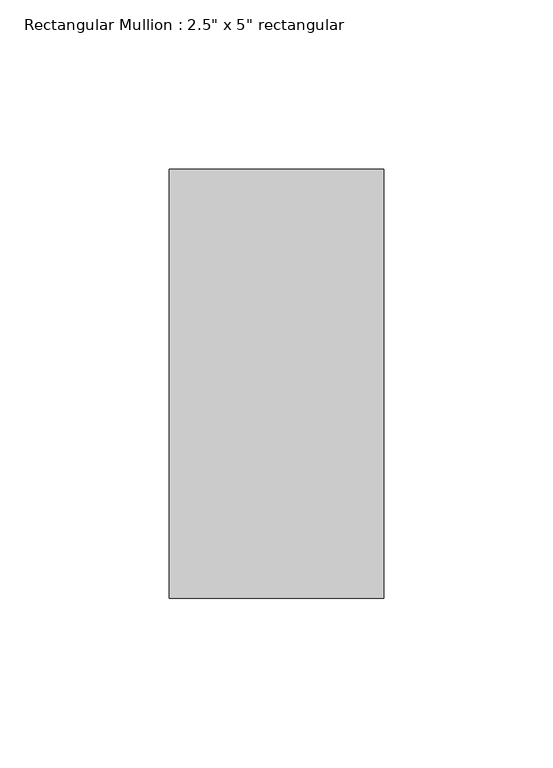
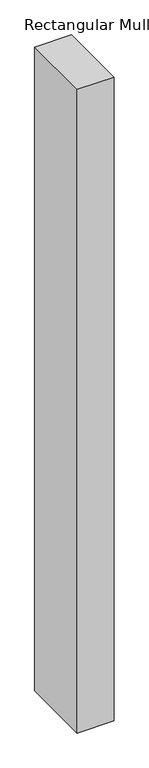
"""IFC4 building model written with IfcOpenShell, lengths in millimetres: member geometry."""

from ifc_helpers import new_model, si_unit, frame, origin, place, context, project, spatial, polyline, outline, extrude, source, transform, mapped, element, save


def member_7f2c8287(model_context):
    return source(origin(), model_context, "Body", "SweptSolid", [
        extrude(outline(polyline([(31.75, 63.5), (31.75, -63.5), (-31.75, -63.5), (-31.75, 63.5), (31.75, 63.5)])), frame((0.0, 0.0, -1174.7500001), z_axis=(0.0, 0.0, 1.0), x_axis=(1.0, 0.0, 0.0)), (0.0, 0.0, 1.0), 1174.7500001),
    ])


if __name__ == "__main__":
    model = new_model("IFC4")
    model_context = context("Model", 3, world=origin())
    ifc_project = project(units=[si_unit("LENGTHUNIT", "METRE", prefix="MILLI")], contexts=[model_context])
    site = spatial("IfcSite", under=ifc_project)
    building = spatial("IfcBuilding", under=site)
    placement = place(None, origin())
    member_shape = member_7f2c8287(model_context)
    element("IfcMember", 1, ObjectType="Rectangular Mullion : 2.5\" x 5\" rectangular", at=placement, inside=building, context=model_context, shape_type="MappedRepresentation", body=[
        mapped(member_shape, transform((0.0, 0.0, 0.0), x_axis=(1.0, 0.0, 0.0), y_axis=(0.0, 1.0, 0.0), z_axis=(0.0, 0.0, 1.0))),
    ])
    save(model, "model.ifc")

# Revit data of these elements
# Type "Rectangular Mullion : 2.5\" x 5\" rectangular"
#   built-in parameter 1007304 = 0.416667 (stored number, unit not read)
#   built-in parameter 1007301 = 0.104167 (stored number, unit not read)
#   built-in parameter 1007300 = 0.104167 (stored number, unit not read)
# Element 1 (IfcMember, "Rectangular Mullion : 2.5\" x 5\" rectangular")
#   Materials on its faces: "WINDOW FRAMING"
# Materials
#   "WINDOW FRAMING": class "Generic", colour RGB 120 120 120, transparency 0, Cost = 0
